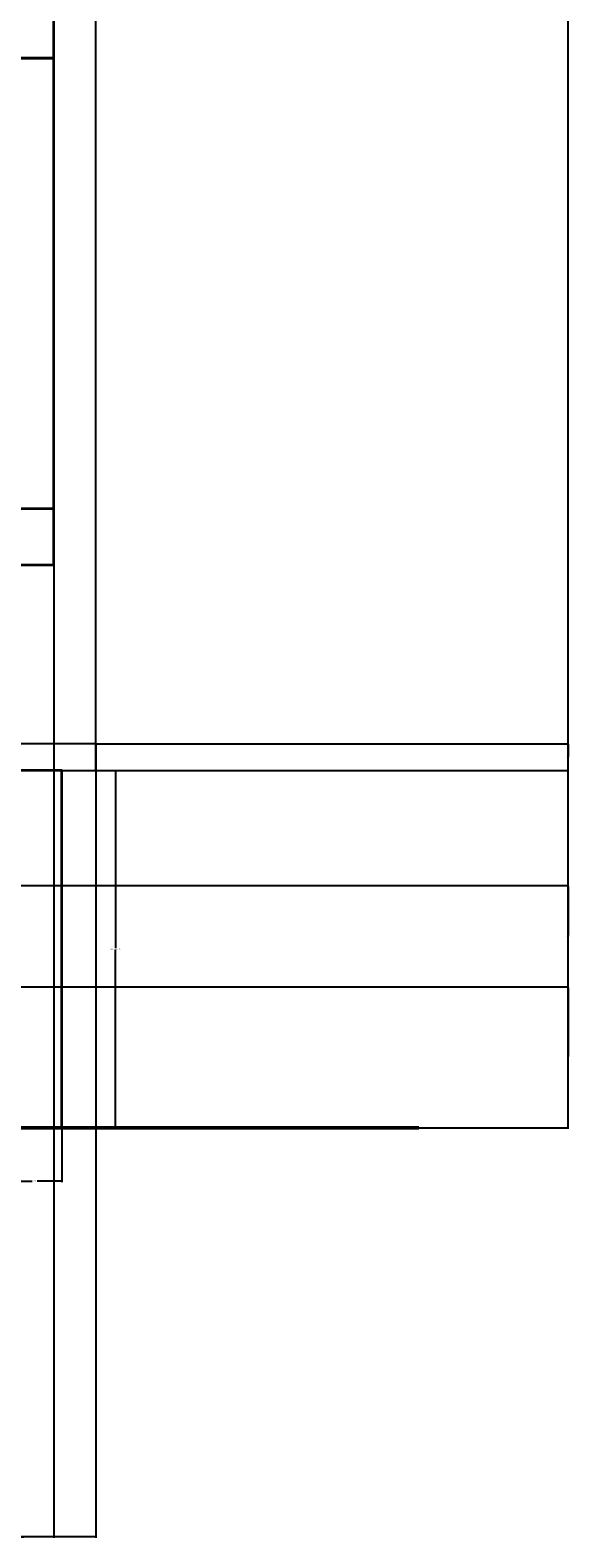
# Model space of a CAD drawing. Units: inches. Extents: x -8 to 554, y -200 to 499.
# Tile 5 of 12: x 439 to 554, y -200 to 121. Entities that reach past the tile are written whole.
import ezdxf

# ---------------------------------------------------------------- set-up
doc = ezdxf.new("R2010")
doc.units = ezdxf.units.IN
doc.header["$MEASUREMENT"] = 0
for name, color, linetype, lineweight in [('A-ANNO-DIMS', 2, 'Continuous', 18), ('A-COLS', 1, 'Continuous', 35), ('A-DOOR-GATE', 3, 'Continuous', 25), ('A-FLOR', 7, 'Continuous', 35), ('A-WALL', 7, 'Continuous', 35), ('C-TOPO', 7, 'Continuous', 50)]:
    doc.layers.add(name, color=color, linetype=linetype, lineweight=lineweight)
doc.styles.get("Standard").update_dxf_attribs({"font": 'arial.ttf'})
doc.dimstyles.get("Standard").update_dxf_attribs({"dimtxt": 0.18, "dimasz": 0.18, "dimexe": 0.18, "dimexo": 0.0625, "dimgap": 0.09, "dimtad": 0, "dimtih": 1, "dimtoh": 1, "dimdec": 4, "dimzin": 0, "dimdsep": 46, "dimtxsty": 'Standard', "dimcen": 0.09, "dimadec": 0, "dimazin": 0, "dimtfac": 1, "dimtdec": 4, "dimtofl": 0, "dimtmove": 0, "dimatfit": 3, "dimfxl": 1, "dimtolj": 1, "dimtzin": 0, "dimarcsym": 0})

# ---------------------------------------------------------------- blocks, each defined once
blk = doc.blocks.new('GATE-PIER-ELEV')
blk.add_lwpolyline([(0, 76.14), (0, 0), (11.66, 0), (11.66, 76.14)])
blk = doc.blocks.new('*D28')
at = {"layer": 'A-ANNO-DIMS', "color": 0, "lineweight": -2, "transparency": 16777216}
for p, q in [((446.15, -36.37), (457.69, -36.37)), ((457.51, -36.55), (457.51, -74.26)), ((457.51, -112.34), (457.51, -74.63)), ((446.15, -112.52), (457.69, -112.52))]:
    blk.add_line(p, q, dxfattribs=at)
at = {"layer": 'A-ANNO-DIMS', "color": 0, "transparency": 16777216}
for points in [[(457.48, -36.55), (457.54, -36.55), (457.51, -36.37)], [(457.48, -112.34), (457.54, -112.34), (457.51, -112.52)]]:
    blk.add_solid(points, dxfattribs=at)
at = {"layer": 'Defpoints', "color": 0, "transparency": 16777216}
for p in [(446.09, -36.37), (446.09, -112.52), (457.51, -112.52)]:
    blk.add_point(p, dxfattribs=at)
at = {"layer": 'A-ANNO-DIMS', "color": 0, "transparency": 16777216, "insert": (457.51, -74.45), "char_height": 0.18, "attachment_point": 5}
blk.add_mtext('\\A1;GATE PIER 76 TYP.', dxfattribs=at)
blk = doc.blocks.new('*D29')
at = {"layer": 'A-ANNO-DIMS', "color": 0, "lineweight": -2, "transparency": 16777216}
for p, q in [((434.42, -112.58), (434.42, -124.12)), ((446.09, -112.58), (446.09, -124.12)), ((434.6, -123.94), (439.73, -123.94)), ((445.91, -123.94), (440.77, -123.94))]:
    blk.add_line(p, q, dxfattribs=at)
at = {"layer": 'A-ANNO-DIMS', "color": 0, "transparency": 16777216}
for points in [[(434.6, -123.91), (434.6, -123.97), (434.42, -123.94)], [(445.91, -123.91), (445.91, -123.97), (446.09, -123.94)]]:
    blk.add_solid(points, dxfattribs=at)
at = {"layer": 'Defpoints', "color": 0, "transparency": 16777216}
for p in [(434.42, -112.52), (446.09, -112.52), (434.42, -123.94)]:
    blk.add_point(p, dxfattribs=at)
at = {"layer": 'A-ANNO-DIMS', "color": 0, "transparency": 16777216, "insert": (440.25, -123.94), "char_height": 0.18, "attachment_point": 5}
blk.add_mtext('\\A1;12 TYP.', dxfattribs=at)
blk = doc.blocks.new('*D30')
at = {"layer": 'A-ANNO-DIMS', "color": 0, "lineweight": -2, "transparency": 16777216}
for p, q in [((444.4, 439.48), (554.26, 439.48)), ((554.08, 439.3), (554.08, 163.66)), ((554.08, -112.34), (554.08, 163.3)), ((446.15, -112.52), (554.26, -112.52))]:
    blk.add_line(p, q, dxfattribs=at)
at = {"layer": 'A-ANNO-DIMS', "color": 0, "transparency": 16777216}
for points in [[(554.05, 439.3), (554.11, 439.3), (554.08, 439.48)], [(554.05, -112.34), (554.11, -112.34), (554.08, -112.52)]]:
    blk.add_solid(points, dxfattribs=at)
at = {"layer": 'Defpoints', "color": 0, "transparency": 16777216}
for p in [(444.34, 439.48), (446.09, -112.52), (554.08, -112.52)]:
    blk.add_point(p, dxfattribs=at)
at = {"layer": 'A-ANNO-DIMS', "color": 0, "transparency": 16777216, "insert": (554.08, 163.48), "char_height": 0.18, "attachment_point": 5}
blk.add_mtext('\\A1;552', dxfattribs=at)
blk = doc.blocks.new('*D31')
at = {"layer": 'A-ANNO-DIMS', "color": 0, "lineweight": -2, "transparency": 16777216}
for p, q in [((24.34, 127.42), (24.34, -199.97)), ((453.32, -30.73), (453.32, -199.97)), ((24.52, -199.79), (238.54, -199.79)), ((453.14, -199.79), (239.12, -199.79))]:
    blk.add_line(p, q, dxfattribs=at)
at = {"layer": 'A-ANNO-DIMS', "color": 0, "transparency": 16777216}
for points in [[(24.52, -199.76), (24.52, -199.82), (24.34, -199.79)], [(453.14, -199.76), (453.14, -199.82), (453.32, -199.79)]]:
    blk.add_solid(points, dxfattribs=at)
at = {"layer": 'Defpoints', "color": 0, "transparency": 16777216}
for p in [(24.34, 127.48), (453.32, -30.67), (453.32, -199.79)]:
    blk.add_point(p, dxfattribs=at)
at = {"layer": 'A-ANNO-DIMS', "color": 0, "transparency": 16777216, "insert": (238.83, -199.79), "char_height": 0.18, "attachment_point": 5}
blk.add_mtext('\\A1;429', dxfattribs=at)
blk = doc.blocks.new('*D32')
at = {"layer": 'A-ANNO-DIMS', "color": 0, "lineweight": -2, "transparency": 16777216}
for p, q in [((24.34, 223.42), (24.34, -199.97)), ((444.34, 223.42), (444.34, -199.97)), ((24.52, -199.79), (234.05, -199.79)), ((444.16, -199.79), (234.63, -199.79))]:
    blk.add_line(p, q, dxfattribs=at)
at = {"layer": 'A-ANNO-DIMS', "color": 0, "transparency": 16777216}
for points in [[(24.52, -199.76), (24.52, -199.82), (24.34, -199.79)], [(444.16, -199.76), (444.16, -199.82), (444.34, -199.79)]]:
    blk.add_solid(points, dxfattribs=at)
at = {"layer": 'Defpoints', "color": 0, "transparency": 16777216}
for p in [(24.34, 223.48), (444.34, 223.48), (444.34, -199.79)]:
    blk.add_point(p, dxfattribs=at)
at = {"layer": 'A-ANNO-DIMS', "color": 0, "transparency": 16777216, "insert": (234.34, -199.79), "char_height": 0.18, "attachment_point": 5}
blk.add_mtext('\\A1;420', dxfattribs=at)
blk = doc.blocks.new('*D55')
at = {"layer": 'A-ANNO-DIMS', "color": 0, "lineweight": -2, "transparency": 16777216}
for p, q in [((204.61, -30.61), (204.61, 498.99)), ((204.79, 498.81), (328.57, 498.81)), ((453.14, 498.81), (329.36, 498.81)), ((453.32, -30.61), (453.32, 498.99))]:
    blk.add_line(p, q, dxfattribs=at)
at = {"layer": 'A-ANNO-DIMS', "color": 0, "transparency": 16777216}
for points in [[(204.79, 498.84), (204.79, 498.78), (204.61, 498.81)], [(453.14, 498.84), (453.14, 498.78), (453.32, 498.81)]]:
    blk.add_solid(points, dxfattribs=at)
at = {"layer": 'Defpoints', "color": 0, "transparency": 16777216}
for p in [(453.32, 498.81), (204.61, -30.67), (453.32, -30.67)]:
    blk.add_point(p, dxfattribs=at)
at = {"layer": 'A-ANNO-DIMS', "color": 0, "transparency": 16777216, "insert": (328.96, 498.81), "char_height": 0.18, "attachment_point": 5}
blk.add_mtext('\\A1;248.7', dxfattribs=at)
blk = doc.blocks.new('*D71')
at = {"layer": 'A-ANNO-DIMS', "color": 0, "lineweight": -2, "transparency": 16777216}
for p, q in [((444.34, 439.42), (444.34, -199.97)), ((432.52, 427.42), (432.52, -199.97)), ((432.7, -199.79), (437.97, -199.79)), ((444.16, -199.79), (438.89, -199.79))]:
    blk.add_line(p, q, dxfattribs=at)
at = {"layer": 'A-ANNO-DIMS', "color": 0, "transparency": 16777216}
for points in [[(432.7, -199.76), (432.7, -199.82), (432.52, -199.79)], [(444.16, -199.76), (444.16, -199.82), (444.34, -199.79)]]:
    blk.add_solid(points, dxfattribs=at)
at = {"layer": 'Defpoints', "color": 0, "transparency": 16777216}
for p in [(444.34, 439.48), (432.52, 427.48), (444.34, -199.79)]:
    blk.add_point(p, dxfattribs=at)
at = {"layer": 'A-ANNO-DIMS', "color": 0, "transparency": 16777216, "insert": (438.43, -199.79), "char_height": 0.18, "attachment_point": 5}
blk.add_mtext('\\A1;11.825', dxfattribs=at)
blk = doc.blocks.new('*D76')
at = {"layer": 'A-ANNO-DIMS', "color": 0, "lineweight": -2, "transparency": 16777216}
for p, q in [((48.75, -82.52), (554.26, -82.52)), ((554.08, -82.7), (554.08, -97.34)), ((554.08, -112.34), (554.08, -97.7)), ((48.75, -112.52), (554.26, -112.52))]:
    blk.add_line(p, q, dxfattribs=at)
at = {"layer": 'A-ANNO-DIMS', "color": 0, "transparency": 16777216}
for points in [[(554.05, -82.7), (554.11, -82.7), (554.08, -82.52)], [(554.05, -112.34), (554.11, -112.34), (554.08, -112.52)]]:
    blk.add_solid(points, dxfattribs=at)
at = {"layer": 'Defpoints', "color": 0, "transparency": 16777216}
for p in [(48.69, -82.52), (554.08, -82.52), (48.69, -112.52)]:
    blk.add_point(p, dxfattribs=at)
at = {"layer": 'A-ANNO-DIMS', "color": 0, "transparency": 16777216, "insert": (554.08, -97.52), "char_height": 0.18, "attachment_point": 5}
blk.add_mtext('\\A1;30', dxfattribs=at)
blk = doc.blocks.new('*D77')
at = {"layer": 'A-ANNO-DIMS', "color": 0, "lineweight": -2, "transparency": 16777216}
for p, q in [((48.75, -60.9), (554.26, -60.9)), ((554.08, -61.08), (554.08, -71.53)), ((554.08, -82.34), (554.08, -71.89)), ((48.75, -82.52), (554.26, -82.52))]:
    blk.add_line(p, q, dxfattribs=at)
at = {"layer": 'A-ANNO-DIMS', "color": 0, "transparency": 16777216}
for points in [[(554.05, -61.08), (554.11, -61.08), (554.08, -60.9)], [(554.05, -82.34), (554.11, -82.34), (554.08, -82.52)]]:
    blk.add_solid(points, dxfattribs=at)
at = {"layer": 'Defpoints', "color": 0, "transparency": 16777216}
for p in [(48.69, -60.9), (554.08, -60.9), (48.69, -82.52)]:
    blk.add_point(p, dxfattribs=at)
at = {"layer": 'A-ANNO-DIMS', "color": 0, "transparency": 16777216, "insert": (554.08, -71.71), "char_height": 0.18, "attachment_point": 5}
blk.add_mtext('\\A1;21.615', dxfattribs=at)
blk = doc.blocks.new('*D78')
at = {"layer": 'A-ANNO-DIMS', "color": 0, "lineweight": -2, "transparency": 16777216}
for p, q in [((453.38, -30.67), (554.26, -30.67)), ((554.08, -30.85), (554.08, -33.34)), ((554.08, -36.19), (554.08, -33.7)), ((453.38, -36.37), (554.26, -36.37))]:
    blk.add_line(p, q, dxfattribs=at)
at = {"layer": 'A-ANNO-DIMS', "color": 0, "transparency": 16777216}
for points in [[(554.05, -30.85), (554.11, -30.85), (554.08, -30.67)], [(554.05, -36.19), (554.11, -36.19), (554.08, -36.37)]]:
    blk.add_solid(points, dxfattribs=at)
at = {"layer": 'Defpoints', "color": 0, "transparency": 16777216}
for p in [(453.32, -30.67), (453.32, -36.37), (554.08, -36.37)]:
    blk.add_point(p, dxfattribs=at)
at = {"layer": 'A-ANNO-DIMS', "color": 0, "transparency": 16777216, "insert": (554.08, -33.52), "char_height": 0.18, "attachment_point": 5}
blk.add_mtext('\\A1;5.706', dxfattribs=at)

msp = doc.modelspace()

# ---------------------------------------------------------------- linework, layer by layer
at = {"layer": 'A-DOOR-GATE'}
msp.add_lwpolyline([(446.0855, -36.3739), (453.3222, -36.3739), (453.3222, -30.6677), (204.6055, -30.6677), (204.6055, -36.3739), (212.2282, -36.3739)], dxfattribs=at)
at = {"layer": 'A-FLOR'}
for p, q in [((24.3421, 115.4814), (444.3421, 115.4814)), ((444.3421, 115.4814), (36.3421, 115.4814)), ((36.3421, 19.4814), (444.3421, 19.4814)), ((24.3421, 7.4814), (444.3421, 7.4814))]:
    msp.add_line(p, q, dxfattribs=at)
at = {"layer": 'A-WALL'}
for p, q in [((444.3421, 115.4814), (444.3421, 235.4814)), ((444.3421, 7.4814), (444.3421, 127.4814))]:
    msp.add_line(p, q, dxfattribs=at)
at = {"layer": 'C-TOPO'}
msp.add_line((24.3421, -112.5186), (522.2333, -112.5186), dxfattribs=at)

# ---------------------------------------------------------------- block references
at = {"layer": 'A-COLS', "rotation": 180}
msp.add_blockref('GATE-PIER-ELEV', (446.0855, -36.3739), dxfattribs=at)

# ---------------------------------------------------------------- dimensions: what is measured, and where the dimension line sits
at = {"layer": 'A-ANNO-DIMS'}
for base, p1, p2, override, picture, middle in [((453.3222, 498.8091), (204.6055, -30.6677), (453.3222, -30.6677), {"dimdec": 1, "dimlfac": 1, "dimrnd": 0, "dimzin": 0, "dimdsep": 46, "dimlunit": 2}, '*D55', (328.9639, 498.8091)), ((444.3421, -199.7912), (432.5174, 427.4814), (444.3421, 439.4814), {"dimdec": 3, "dimlfac": 1, "dimrnd": 0, "dimzin": 0, "dimdsep": 46, "dimlunit": 2}, '*D71', (438.4297, -199.7912)), ((444.3421, -199.7912), (24.3421, 223.4814), (444.3421, 223.4814), {"dimdec": 0, "dimlfac": 1, "dimrnd": 0, "dimzin": 0, "dimdsep": 46, "dimlunit": 2}, '*D32', (234.3421, -199.7912)), ((453.3222, -199.7912), (24.3421, 127.4814), (453.3222, -30.6677), {"dimdec": 0, "dimlfac": 1, "dimrnd": 0, "dimzin": 0, "dimdsep": 46, "dimlunit": 2}, '*D31', (238.8321, -199.7912))]:
    dim = msp.add_linear_dim(base=base, p1=p1, p2=p2, dimstyle='Standard', override=override, dxfattribs=at)
    dim.commit()
    dim.dimension.update_dxf_attribs({"geometry": picture, "text_midpoint": middle})
for base, p1, p2, override, picture, middle in [((554.0833, -112.5186), (444.3421, 439.4814), (446.0855, -112.5186), {"dimdec": 0, "dimlfac": 1, "dimrnd": 0, "dimzin": 0, "dimdsep": 46, "dimlunit": 2}, '*D30', (554.0833, 163.4814)), ((554.0833, -36.3739), (453.3222, -30.6677), (453.3222, -36.3739), {"dimdec": 3, "dimlfac": 1, "dimrnd": 0, "dimzin": 0, "dimdsep": 46, "dimlunit": 2}, '*D78', (554.0833, -33.5208)), ((554.0833, -60.9032), (48.6882, -82.5186), (48.6882, -60.9032), {"dimdec": 3, "dimlfac": 1, "dimrnd": 0, "dimzin": 0, "dimdsep": 46, "dimlunit": 2}, '*D77', (554.0833, -71.7109)), ((554.0833, -82.5186), (48.6882, -112.5186), (48.6882, -82.5186), {"dimdec": 0, "dimlfac": 1, "dimrnd": 0, "dimzin": 0, "dimdsep": 46, "dimlunit": 2}, '*D76', (554.0833, -97.5186))]:
    dim = msp.add_linear_dim(base=base, p1=p1, p2=p2, angle=90, dimstyle='Standard', override=override, dxfattribs=at)
    dim.commit()
    dim.dimension.update_dxf_attribs({"geometry": picture, "text_midpoint": middle})
for base, p1, p2, angle, text, picture, middle in [((457.5072, -112.5186), (446.0855, -36.3739), (446.0855, -112.5186), 270, 'GATE PIER <> TYP.', '*D28', (457.5072, -74.4463)), ((434.4225, -123.9404), (446.0855, -112.5186), (434.4225, -112.5186), 180, '<> TYP.', '*D29', (440.254, -123.9404))]:
    dim = msp.add_linear_dim(base=base, p1=p1, p2=p2, angle=angle, text=text, dimstyle='Standard', override={"dimdec": 0, "dimlfac": 1, "dimrnd": 0, "dimzin": 0, "dimdsep": 46, "dimlunit": 2}, dxfattribs=at)
    dim.commit()
    dim.dimension.update_dxf_attribs({"geometry": picture, "text_midpoint": middle})

doc.saveas('drawing.dxf')
